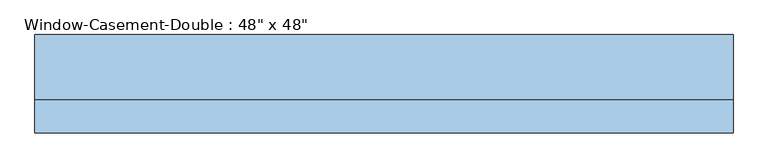
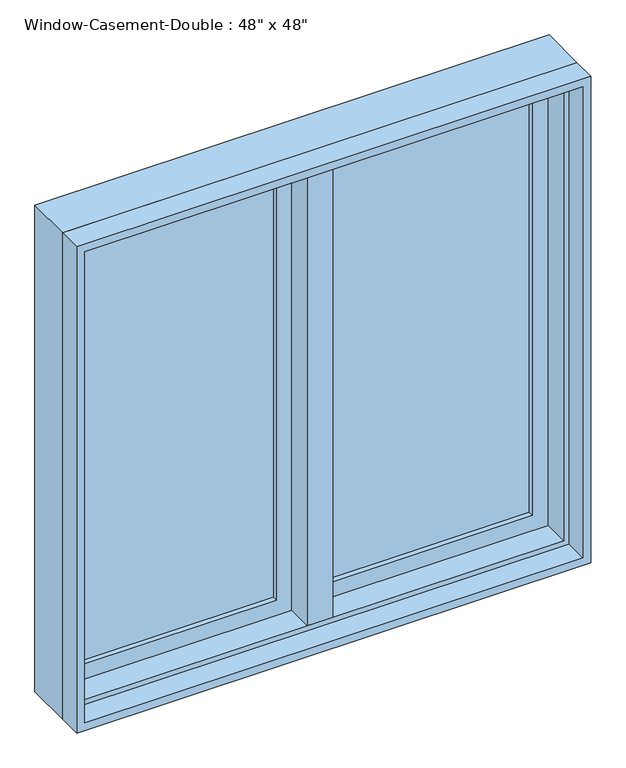
"""IFC4 building model written with IfcOpenShell, lengths in millimetres: window geometry."""

from ifc_helpers import new_model, si_unit, frame, origin, place, context, project, spatial, polyline, outline, extrude, faceted_brep, source, transform, mapped, element, save


def window_191d0cfb(model_context):
    return source(origin(), model_context, "Body", "SolidModel", [
        faceted_brep([(9.525, 95.25, 2120.9), (-9.525, 95.25, 2120.9), (-9.525, 44.45, 2120.9), (9.525, 44.45, 2120.9), (9.525, 95.25, 927.1), (9.525, 44.45, 927.1), (-9.525, 44.45, 927.1), (-9.525, 95.25, 927.1), (-9.525, 44.45, 946.15), (-9.525, 44.45, 2101.85), (-30.1625, 44.45, 946.15), (-30.1625, 44.45, 2101.85), (-30.1625, -19.05, 946.15), (-30.1625, -19.05, 2101.85), (30.1625, -19.05, 946.15), (30.1625, -19.05, 2101.85), (30.1625, 44.45, 946.15), (30.1625, 44.45, 2101.85), (9.525, 44.45, 946.15), (9.525, 44.45, 2101.85)], [[[0, 1, 2, 3]], [[4, 5, 6, 7]], [[1, 0, 4, 7]], [[2, 1, 7, 6, 8, 9]], [[9, 8, 10, 11]], [[11, 10, 12, 13]], [[13, 12, 14, 15]], [[15, 14, 16, 17]], [[17, 16, 18, 19]], [[0, 3, 19, 18, 5, 4]], [[18, 8, 6, 5]], [[9, 19, 3, 2]], [[8, 18, 16, 14, 12, 10]], [[19, 9, 11, 13, 15, 17]]]),
        extrude(outline(polyline([(-66.675, 76.2), (-66.675, 69.85), (-539.75, 69.85), (-539.75, 76.2), (-66.675, 76.2)])), frame((0.0, 0.0, 984.25), z_axis=(0.0, 0.0, 1.0), x_axis=(1.0, 0.0, 0.0)), (0.0, 0.0, 1.0), 1079.5),
        extrude(outline(polyline([(-539.75, 57.15), (-539.75, 63.5), (-66.675, 63.5), (-66.675, 57.15), (-539.75, 57.15)])), frame((0.0, 0.0, 984.25), z_axis=(0.0, 0.0, 1.0), x_axis=(1.0, 0.0, 0.0)), (0.0, 0.0, 1.0), 1079.5),
        extrude(outline(polyline([(539.75, 76.2), (539.75, 69.85), (66.675, 69.85), (66.675, 76.2), (539.75, 76.2)])), frame((0.0, 0.0, 984.25), z_axis=(0.0, 0.0, 1.0), x_axis=(1.0, 0.0, 0.0)), (0.0, 0.0, 1.0), 1079.5),
        extrude(outline(polyline([(66.675, 57.15), (66.675, 63.5), (539.75, 63.5), (539.75, 57.15), (66.675, 57.15)])), frame((0.0, 0.0, 984.25), z_axis=(0.0, 0.0, 1.0), x_axis=(1.0, 0.0, 0.0)), (0.0, 0.0, 1.0), 1079.5),
        extrude(outline(polyline([(2120.9, -596.9), (927.1, -596.9), (927.1, -9.525), (2120.9, -9.525), (2120.9, -596.9)]), holes=[polyline([(2063.75, -66.675), (984.25, -66.675), (984.25, -539.75), (2063.75, -539.75), (2063.75, -66.675)])]), frame((0.0, 44.45, 0.0), z_axis=(0.0, 1.0, 0.0), x_axis=(0.0, 0.0, 1.0)), (0.0, 0.0, 1.0), 44.45),
        extrude(outline(polyline([(927.1, 596.9), (2120.9, 596.9), (2120.9, 9.525), (927.1, 9.525), (927.1, 596.9)]), holes=[polyline([(984.25, 66.675), (2063.75, 66.675), (2063.75, 539.75), (984.25, 539.75), (984.25, 66.675)])]), frame((0.0, 44.45, 0.0), z_axis=(0.0, 1.0, 0.0), x_axis=(0.0, 0.0, 1.0)), (0.0, 0.0, 1.0), 44.45),
        extrude(outline(polyline([(2133.6, -609.6), (914.4, -609.6), (914.4, 609.6), (2133.6, 609.6), (2133.6, -609.6)]), holes=[polyline([(2114.55, 590.55), (933.45, 590.55), (933.45, -590.55), (2114.55, -590.55), (2114.55, 590.55)])]), frame((0.0, -76.2, 0.0), z_axis=(0.0, 1.0, 0.0), x_axis=(0.0, 0.0, 1.0)), (0.0, 0.0, 1.0), 57.15),
        faceted_brep([(577.85, 44.45, 2101.85), (577.85, -19.05, 2101.85), (-577.85, -19.05, 2101.85), (-577.85, 44.45, 2101.85), (596.9, 95.25, 2120.9), (596.9, 44.45, 2120.9), (-596.9, 44.45, 2120.9), (-596.9, 95.25, 2120.9), (609.6, -19.05, 2133.6), (609.6, 95.25, 2133.6), (-609.6, 95.25, 2133.6), (-609.6, -19.05, 2133.6), (-577.85, -19.05, 946.15), (-577.85, 44.45, 946.15), (-596.9, 44.45, 927.1), (-596.9, 95.25, 927.1), (-609.6, 95.25, 914.4), (-609.6, -19.05, 914.4), (577.85, -19.05, 946.15), (577.85, 44.45, 946.15), (596.9, 44.45, 927.1), (596.9, 95.25, 927.1), (609.6, 95.25, 914.4), (609.6, -19.05, 914.4)], [[[0, 1, 2, 3]], [[4, 5, 6, 7]], [[8, 9, 10, 11]], [[3, 2, 12, 13]], [[7, 6, 14, 15]], [[11, 10, 16, 17]], [[13, 12, 18, 19]], [[15, 14, 20, 21]], [[17, 16, 22, 23]], [[11, 17, 23, 8], [1, 18, 12, 2]], [[19, 18, 1, 0]], [[5, 20, 14, 6], [3, 13, 19, 0]], [[21, 20, 5, 4]], [[23, 22, 9, 8]], [[9, 22, 16, 10], [7, 15, 21, 4]]]),
    ])


if __name__ == "__main__":
    model = new_model("IFC4")
    model_context = context("Model", 3, world=origin())
    ifc_project = project(units=[si_unit("LENGTHUNIT", "METRE", prefix="MILLI")], contexts=[model_context])
    site = spatial("IfcSite", under=ifc_project)
    building = spatial("IfcBuilding", under=site)
    placement = place(None, origin())
    window_shape = window_191d0cfb(model_context)
    element("IfcWindow", 1, ObjectType="Window-Casement-Double : 48\" x 48\"", at=placement, inside=building, context=model_context, shape_type="MappedRepresentation", body=[
        mapped(window_shape, transform((0.0, 0.0, 0.0), x_axis=(1.0, 0.0, 0.0), y_axis=(0.0, 1.0, 0.0), z_axis=(0.0, 0.0, 1.0))),
    ])
    save(model, "model.ifc")

# Revit data of these elements
# Type "Window-Casement-Double : 48\" x 48\""
#   Type Mark = "16"
#   Fire Rating = "0.5h"
#   Assembly Code = "B2020100"
#   Analytic Construction = "Double glazing - domestic"
#   Frame Extension [instance default] = 0' - 0 1/4"
#   Window Inset [instance default] = 0' - 0"
#   Wall Thickness [instance default] = 0' - 6"
#   Interior Wall Closure [instance default] = 0' - 2 1/4"
#   Half Width = 2' - 0"
#   Visual Light Transmittance = 0.81
#   Thermal Resistance (R) = 1.8146 (h·ft²·°F)/BTU
#   Solar Heat Gain Coefficient = 0.76
#   Rough Width = 4' - 0 1/2"
#   Rough Height = 4' - 0 1/2"
#   Height = 4' - 0"
#   Heat Transfer Coefficient (U) = 0.5511 BTU/(h·ft²·°F)
#   Exterior Wall Closure [instance default] = 0' - 1 1/4"
#   Extension Jamb [instance default] = 0' - 2 1/4"
#   Default Sill Height = 3' - 0"
#   Width = 4' - 0"
#   Define Thermal Properties by = 0
#   Muntin Visibility = yes
#   Interior Trim Visibility [instance default] = yes
#   Exterior Trim Visibility [instance default] = yes
#   Extension Jamb Visibility [instance default] = yes
#   Interior Trim Material = Wood - Stained
#   Muntin Pattern = Muntin Pattern_2x2 : Muntin Pattern_2x2
#   Interior Trim = Trim-Window-Interior-Flat : Picture Frame
#   Interior Frame Material = Wood - Stained
#   Glass Panel Material = Glass
#   Exterior Trim Material = Clad - White
#   Exterior Trim = Trim-Window-Exterior-Flat : with Sill
#   Exterior Frame Material = Clad - White
#   Wall Closure = (empty or 0)
# Element 1 (IfcWindow, "Window-Casement-Double : 48\" x 48\"")
#   Materials on its faces: "Wood - Stained", "Glass", "Clad - White"
# Materials
#   "Wood - Stained": class "Wood", colour RGB 224 178 126, transparency 0, Cost = 0
#   "Glass": class "Glass", colour RGB 0 128 192, transparency 0.75, Description = "Soda Lime Glass", Cost = 0
#   "Clad - White": class "Wood", colour RGB 242 242 238, transparency 0, Cost = 0
